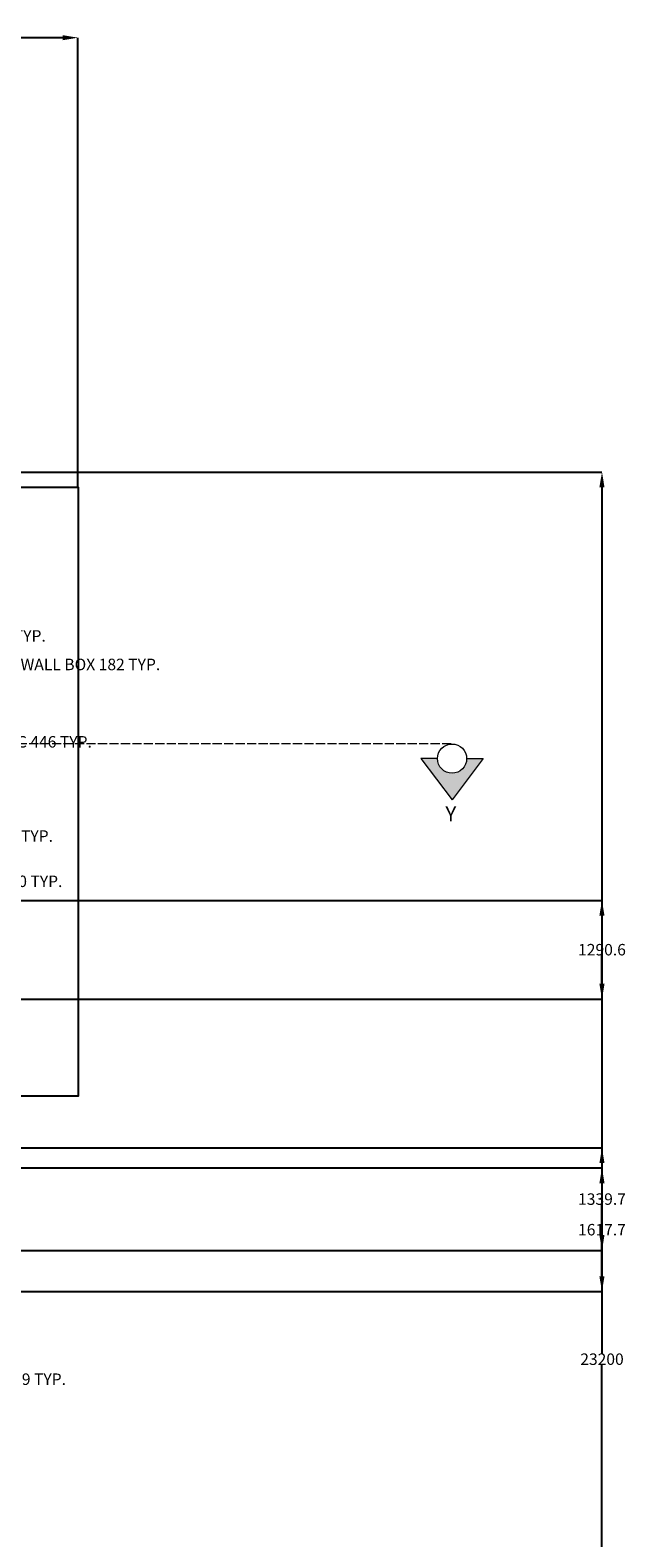
# Model space of a CAD drawing. Units: inches. Extents: x 22626 to 57351, y 2118 to 36234.
# Tile 10 of 10: x 49561 to 57351, y 16521 to 36234. Entities that reach past the tile are written whole.
import ezdxf

# ---------------------------------------------------------------- set-up
doc = ezdxf.new("R2010")
doc.units = ezdxf.units.IN
doc.header["$MEASUREMENT"] = 0
doc.linetypes.add('ACAD_ISO02W100', pattern=[15, 12, -3])
for name, color, linetype, lineweight in [('A-ANNO-DIMS', 130, 'Continuous', 18), ('A-ANNO-SYMB', 130, 'Continuous', 18), ('A-ROOF', 80, 'Continuous', 25)]:
    doc.layers.add(name, color=color, linetype=linetype, lineweight=lineweight)
doc.layers.add('A-SECT', color=2, linetype='ACAD_ISO02W100', lineweight=18, true_color=0xf1eb1f)
doc.styles.get("Standard").update_dxf_attribs({"font": 'arial.ttf'})
doc.dimstyles.get("Standard").update_dxf_attribs({"dimtxt": 150, "dimasz": 200, "dimexe": 0.18, "dimexo": 0.0625, "dimgap": 0.09, "dimtad": 0, "dimtih": 1, "dimtoh": 1, "dimdec": 0, "dimzin": 0, "dimdsep": 46, "dimtxsty": 'Standard', "dimcen": 0.09, "dimadec": 0, "dimazin": 0, "dimtfac": 1, "dimtdec": 0, "dimtofl": 0, "dimtmove": 0, "dimatfit": 3, "dimfxl": 1, "dimtolj": 1, "dimtzin": 0, "dimarcsym": 0})

# ---------------------------------------------------------------- blocks, each defined once
blk = doc.blocks.new('SECTION-HEAD')
h = blk.add_hatch(color=256)
h.dxf.hatch_style = 1
h.paths.add_polyline_path([(815, 541), (599, 541, -1), (216, 541), (0, 541), (407, 0)])
for p, q in [((216, 541), (0, 541)), ((0, 541), (407, 0)), ((815, 541), (407, 0)), ((599, 541), (815, 541))]:
    blk.add_line(p, q)
blk.add_circle((407, 541), 191)
blk = doc.blocks.new('*D62')
at = {"layer": 'A-ANNO-DIMS', "color": 0, "lineweight": -2, "transparency": 16777216}
for p, q in [((48512, 26995), (48512, 26928)), ((48712, 26929), (48757, 26929)), ((48957, 26995), (48957, 26928)), ((48957, 26929), (49157, 26929))]:
    blk.add_line(p, q, dxfattribs=at)
at = {"layer": 'A-ANNO-DIMS', "color": 0, "transparency": 16777216}
for points in [[(48712, 26962), (48712, 26895), (48512, 26929)], [(48757, 26962), (48757, 26895), (48957, 26929)]]:
    blk.add_solid(points, dxfattribs=at)
at = {"layer": 'Defpoints', "color": 0, "transparency": 16777216}
for p in [(48512, 26995), (48957, 26995), (48957, 26929)]:
    blk.add_point(p, dxfattribs=at)
at = {"layer": 'A-ANNO-DIMS', "color": 0, "transparency": 16777216, "insert": (49788, 26929), "char_height": 150, "attachment_point": 5}
blk.add_mtext('\\A1;WC 446 TYP.', dxfattribs=at)
blk = doc.blocks.new('*D64')
at = {"layer": 'A-ANNO-DIMS', "color": 0, "lineweight": -2, "transparency": 16777216}
for p, q in [((48957, 26152), (49094, 26152)), ((49094, 25952), (49094, 25774)), ((49094, 25442), (49094, 25620)), ((48957, 25242), (49094, 25242))]:
    blk.add_line(p, q, dxfattribs=at)
at = {"layer": 'A-ANNO-DIMS', "color": 0, "transparency": 16777216}
for points in [[(49061, 25952), (49127, 25952), (49094, 26152)], [(49061, 25442), (49127, 25442), (49094, 25242)]]:
    blk.add_solid(points, dxfattribs=at)
at = {"layer": 'Defpoints', "color": 0, "transparency": 16777216}
for p in [(48957, 26152), (49094, 26152), (48957, 25242)]:
    blk.add_point(p, dxfattribs=at)
at = {"layer": 'A-ANNO-DIMS', "color": 0, "transparency": 16777216, "insert": (49094, 25697), "char_height": 150, "attachment_point": 5}
blk.add_mtext('\\A1;VANITY 910 TYP.', dxfattribs=at)
blk = doc.blocks.new('*D65')
at = {"layer": 'A-ANNO-DIMS', "color": 0, "lineweight": -2, "transparency": 16777216}
for p, q in [((48348, 25242), (48348, 25105)), ((48957, 25242), (48957, 25105)), ((48548, 25105), (48757, 25105)), ((48957, 25105), (49157, 25105))]:
    blk.add_line(p, q, dxfattribs=at)
at = {"layer": 'A-ANNO-DIMS', "color": 0, "transparency": 16777216}
for points in [[(48548, 25139), (48548, 25072), (48348, 25105)], [(48757, 25139), (48757, 25072), (48957, 25105)]]:
    blk.add_solid(points, dxfattribs=at)
at = {"layer": 'Defpoints', "color": 0, "transparency": 16777216}
for p in [(48348, 25242), (48957, 25242), (48957, 25105)]:
    blk.add_point(p, dxfattribs=at)
at = {"layer": 'A-ANNO-DIMS', "color": 0, "transparency": 16777216, "insert": (49581, 25105), "char_height": 150, "attachment_point": 5}
blk.add_mtext('\\A1;610 TYP.', dxfattribs=at)
blk = doc.blocks.new('*D66')
at = {"layer": 'A-ANNO-DIMS', "color": 0, "lineweight": -2, "transparency": 16777216}
for p, q in [((46732, 18595), (46532, 18595)), ((46932, 18567), (46932, 18595)), ((47122, 18567), (47122, 18595)), ((47322, 18595), (47522, 18595))]:
    blk.add_line(p, q, dxfattribs=at)
at = {"layer": 'A-ANNO-DIMS', "color": 0, "transparency": 16777216}
for points in [[(46732, 18629), (46732, 18562), (46932, 18595)], [(47322, 18629), (47322, 18562), (47122, 18595)]]:
    blk.add_solid(points, dxfattribs=at)
at = {"layer": 'Defpoints', "color": 0, "transparency": 16777216}
for p in [(46932, 18567), (47122, 18595), (47122, 18567)]:
    blk.add_point(p, dxfattribs=at)
at = {"layer": 'A-ANNO-DIMS', "color": 0, "transparency": 16777216, "insert": (48824, 18595), "char_height": 150, "attachment_point": 5}
blk.add_mtext('\\A1;SUPPLY FITTING 189 TYP.', dxfattribs=at)
blk = doc.blocks.new('*D70')
at = {"layer": 'A-ANNO-DIMS', "color": 0, "lineweight": -2, "transparency": 16777216}
for p, q in [((48575, 27941), (48375, 27941)), ((48775, 27914), (48775, 27941)), ((48957, 27914), (48957, 27941)), ((49157, 27941), (49357, 27941))]:
    blk.add_line(p, q, dxfattribs=at)
at = {"layer": 'A-ANNO-DIMS', "color": 0, "transparency": 16777216}
for points in [[(48575, 27974), (48575, 27908), (48775, 27941)], [(49157, 27974), (49157, 27908), (48957, 27941)]]:
    blk.add_solid(points, dxfattribs=at)
at = {"layer": 'Defpoints', "color": 0, "transparency": 16777216}
for p in [(48775, 27914), (48957, 27941), (48957, 27914)]:
    blk.add_point(p, dxfattribs=at)
at = {"layer": 'A-ANNO-DIMS', "color": 0, "transparency": 16777216, "insert": (50349, 27941), "char_height": 150, "attachment_point": 5}
blk.add_mtext('\\A1;WALL BOX 182 TYP.', dxfattribs=at)
blk = doc.blocks.new('*D71')
at = {"layer": 'A-ANNO-DIMS', "color": 0, "lineweight": -2, "transparency": 16777216}
for p, q in [((48748, 28114), (48748, 28314)), ((48748, 28314), (48948, 28314)), ((48775, 27914), (48748, 27914)), ((48775, 27807), (48748, 27807)), ((48748, 27607), (48748, 27407))]:
    blk.add_line(p, q, dxfattribs=at)
at = {"layer": 'A-ANNO-DIMS', "color": 0, "transparency": 16777216}
for points in [[(48715, 28114), (48781, 28114), (48748, 27914)], [(48715, 27607), (48781, 27607), (48748, 27807)]]:
    blk.add_solid(points, dxfattribs=at)
at = {"layer": 'Defpoints', "color": 0, "transparency": 16777216}
for p in [(48748, 27914), (48775, 27914), (48775, 27807)]:
    blk.add_point(p, dxfattribs=at)
at = {"layer": 'A-ANNO-DIMS', "color": 0, "transparency": 16777216, "insert": (49364, 28314), "char_height": 150, "attachment_point": 5}
blk.add_mtext('\\A1;107 TYP.', dxfattribs=at)
blk = doc.blocks.new('*D98')
at = {"layer": 'A-ANNO-DIMS', "color": 0, "lineweight": -2, "transparency": 16777216}
for p, q in [((30057, 30257), (30057, 36136)), ((30257, 36136), (39839, 36136)), ((49987, 36136), (40406, 36136)), ((50187, 30257), (50187, 36136))]:
    blk.add_line(p, q, dxfattribs=at)
at = {"layer": 'A-ANNO-DIMS', "color": 0, "transparency": 16777216}
for points in [[(30257, 36169), (30257, 36103), (30057, 36136)], [(49987, 36169), (49987, 36103), (50187, 36136)]]:
    blk.add_solid(points, dxfattribs=at)
at = {"layer": 'Defpoints', "color": 0, "transparency": 16777216}
for p in [(50187, 36136), (30057, 30257), (50187, 30257)]:
    blk.add_point(p, dxfattribs=at)
at = {"layer": 'A-ANNO-DIMS', "color": 0, "transparency": 16777216, "insert": (40122, 36136), "char_height": 150, "attachment_point": 5}
blk.add_mtext('\\A1;20130', dxfattribs=at)
blk = doc.blocks.new('*D99')
at = {"layer": 'A-ANNO-DIMS', "color": 0, "lineweight": -2, "transparency": 16777216}
for p, q in [((41185, 30457), (57039, 30457)), ((57039, 30257), (57039, 18934)), ((57039, 7457), (57039, 18780)), ((43702, 7257), (57039, 7257))]:
    blk.add_line(p, q, dxfattribs=at)
at = {"layer": 'A-ANNO-DIMS', "color": 0, "transparency": 16777216}
for points in [[(57005, 30257), (57072, 30257), (57039, 30457)], [(57005, 7457), (57072, 7457), (57039, 7257)]]:
    blk.add_solid(points, dxfattribs=at)
at = {"layer": 'Defpoints', "color": 0, "transparency": 16777216}
for p in [(41185, 30457), (57039, 30457), (43702, 7257)]:
    blk.add_point(p, dxfattribs=at)
at = {"layer": 'A-ANNO-DIMS', "color": 0, "transparency": 16777216, "insert": (57039, 18857), "char_height": 150, "attachment_point": 5}
blk.add_mtext('\\A1;23200', dxfattribs=at)
blk = doc.blocks.new('*D103')
at = {"layer": 'A-ANNO-DIMS', "color": 0, "lineweight": -2, "transparency": 16777216}
for p, q in [((42816, 21358), (57039, 21358)), ((57039, 21158), (57039, 20626)), ((57039, 19941), (57039, 20473)), ((42816, 19741), (57039, 19741))]:
    blk.add_line(p, q, dxfattribs=at)
at = {"layer": 'A-ANNO-DIMS', "color": 0, "transparency": 16777216}
for points in [[(57005, 21158), (57072, 21158), (57039, 21358)], [(57005, 19941), (57072, 19941), (57039, 19741)]]:
    blk.add_solid(points, dxfattribs=at)
at = {"layer": 'Defpoints', "color": 0, "transparency": 16777216}
for p in [(42816, 21358), (57039, 21358), (42816, 19741)]:
    blk.add_point(p, dxfattribs=at)
at = {"layer": 'A-ANNO-DIMS', "color": 0, "transparency": 16777216, "insert": (57039, 20550), "char_height": 150, "attachment_point": 5}
blk.add_mtext('\\A1;1617.7', dxfattribs=at)
blk = doc.blocks.new('*D105')
at = {"layer": 'A-ANNO-DIMS', "color": 0, "lineweight": -2, "transparency": 16777216}
for p, q in [((39983, 21620), (57039, 21620)), ((57039, 21420), (57039, 21027)), ((57039, 20480), (57039, 20874)), ((39983, 20280), (57039, 20280))]:
    blk.add_line(p, q, dxfattribs=at)
at = {"layer": 'A-ANNO-DIMS', "color": 0, "transparency": 16777216}
for points in [[(57005, 21420), (57072, 21420), (57039, 21620)], [(57005, 20480), (57072, 20480), (57039, 20280)]]:
    blk.add_solid(points, dxfattribs=at)
at = {"layer": 'Defpoints', "color": 0, "transparency": 16777216}
for p in [(39983, 21620), (57039, 21620), (39983, 20280)]:
    blk.add_point(p, dxfattribs=at)
at = {"layer": 'A-ANNO-DIMS', "color": 0, "transparency": 16777216, "insert": (57039, 20950), "char_height": 150, "attachment_point": 5}
blk.add_mtext('\\A1;1339.7', dxfattribs=at)
blk = doc.blocks.new('*D109')
at = {"layer": 'A-ANNO-DIMS', "color": 0, "lineweight": -2, "transparency": 16777216}
for p, q in [((38641, 24856), (57039, 24856)), ((57039, 24656), (57039, 24287)), ((57039, 23765), (57039, 24134)), ((38641, 23565), (57039, 23565))]:
    blk.add_line(p, q, dxfattribs=at)
at = {"layer": 'A-ANNO-DIMS', "color": 0, "transparency": 16777216}
for points in [[(57005, 24656), (57072, 24656), (57039, 24856)], [(57005, 23765), (57072, 23765), (57039, 23565)]]:
    blk.add_solid(points, dxfattribs=at)
at = {"layer": 'Defpoints', "color": 0, "transparency": 16777216}
for p in [(38641, 24856), (57039, 24856), (38641, 23565)]:
    blk.add_point(p, dxfattribs=at)
at = {"layer": 'A-ANNO-DIMS', "color": 0, "transparency": 16777216, "insert": (57039, 24211), "char_height": 150, "attachment_point": 5}
blk.add_mtext('\\A1;1290.6', dxfattribs=at)
blk = doc.blocks.new('*D115')
at = {"layer": 'A-ANNO-DIMS', "color": 0, "lineweight": -2, "transparency": 16777216}
for p, q in [((47973, 25697), (48173, 25697)), ((49783, 25697), (49783, 25697)), ((49783, 25697), (49783, 25697))]:
    blk.add_line(p, q, dxfattribs=at)
at = {"layer": 'A-ANNO-DIMS', "color": 0, "transparency": 16777216}
blk.add_solid([(48173, 25730), (48173, 25664), (48373, 25697)], dxfattribs=at)
at = {"layer": 'Defpoints', "color": 0, "transparency": 16777216}
for p in [(48373, 25697), (49783, 25697)]:
    blk.add_point(p, dxfattribs=at)
at = {"layer": 'A-ANNO-DIMS', "color": 0, "transparency": 16777216, "insert": (47515, 25697), "char_height": 150, "attachment_point": 5}
blk.add_mtext('\\A1;2X R1410', dxfattribs=at)

msp = doc.modelspace()

# ---------------------------------------------------------------- linework, layer by layer
at = {"layer": 'A-ROOF'}
msp.add_lwpolyline([(41184.53, 30256.86), (50187.43, 30256.86), (50187.43, 25126.86), (50187.43, 22296.86), (48682.43, 22296.86), (48682.43, 11956.86), (43702.43, 11956.86)], dxfattribs=at)
at = {"layer": 'A-SECT', "ltscale": 10}
msp.add_line((55067.61, 26900.74), (24870.06, 26900.74), dxfattribs=at)

# ---------------------------------------------------------------- block references
at = {"layer": 'A-ANNO-SYMB'}
msp.add_blockref('SECTION-HEAD', (54671.15, 26168.47), dxfattribs=at)

# ---------------------------------------------------------------- texts
msp.add_text('Y', height=200, dxfattribs=at).set_placement((54989.81, 25887.63))

# ---------------------------------------------------------------- dimensions: what is measured, and where the dimension line sits
at = {"layer": 'A-ANNO-DIMS'}
dim = msp.add_linear_dim(base=(50187.43, 36136.06), p1=(30057.43, 30256.86), p2=(50187.43, 30256.86), dimstyle='Standard', override={"dimdec": 0, "dimlfac": 1, "dimrnd": 0, "dimzin": 0, "dimdsep": 46, "dimlunit": 2}, dxfattribs=at)
dim.commit()
dim.dimension.update_dxf_attribs({"geometry": '*D98', "text_midpoint": (40122.43, 36136.06)})
for base, p1, p2, override, picture, middle in [((57038.61, 30456.86), (43702.43, 7256.86), (41184.53, 30456.86), {"dimdec": 0, "dimlfac": 1, "dimrnd": 0, "dimzin": 0, "dimdsep": 46, "dimlunit": 2}, '*D99', (57038.61, 18856.86)), ((57038.61, 24856.11), (38641.03, 23565.5), (38641.03, 24856.11), {"dimdec": 1, "dimlfac": 1, "dimrnd": 0, "dimzin": 0, "dimdsep": 46, "dimlunit": 2}, '*D109', (57038.61, 24210.8)), ((57038.61, 21620.09), (39982.98, 20280.39), (39982.98, 21620.09), {"dimdec": 1, "dimlfac": 1, "dimrnd": 0, "dimzin": 0, "dimdsep": 46, "dimlunit": 2}, '*D105', (57038.61, 20950.24)), ((57038.6134, 21358.3711), (42815.7406, 19740.7168), (42815.7406, 21358.3711), {"dimdec": 1, "dimlfac": 1, "dimrnd": 0, "dimzin": 0, "dimdsep": 46, "dimlunit": 2}, '*D103', (57038.6134, 20549.5439))]:
    dim = msp.add_linear_dim(base=base, p1=p1, p2=p2, angle=90, dimstyle='Standard', override=override, dxfattribs=at)
    dim.commit()
    dim.dimension.update_dxf_attribs({"geometry": picture, "text_midpoint": middle})
for base, p1, p2, text, picture, middle in [((48957.43, 27941), (48775.41, 27913.69), (48957.43, 27913.69), 'WALL BOX <> TYP.', '*D70', (50348.74, 27941)), ((48957.43, 26928.62), (48511.9, 26995.45), (48957.43, 26995.45), 'WC <> TYP.', '*D62', (49787.6, 26928.62)), ((48957.43, 25105.35), (48347.56, 25241.86), (48957.43, 25241.86), '<> TYP.', '*D65', (49581.27, 25105.35)), ((47121.6, 18595.27), (46932.22, 18566.86), (47121.6, 18566.86), 'SUPPLY FITTING <> TYP.', '*D66', (48823.75, 18595.27))]:
    dim = msp.add_linear_dim(base=base, p1=p1, p2=p2, text=text, dimstyle='Standard', override={"dimdec": 0, "dimlfac": 1, "dimrnd": 0, "dimzin": 0, "dimdsep": 46, "dimlunit": 2}, dxfattribs=at)
    dim.commit()
    dim.dimension.update_dxf_attribs({"geometry": picture, "text_midpoint": middle})
for base, p1, p2, text, picture, middle in [((48748.11, 27913.69), (48775.41, 27806.86), (48775.41, 27913.69), '<> TYP.', '*D71', (49364.48, 28313.69)), ((49093.94, 26151.9), (48957.43, 25241.86), (48957.43, 26151.9), 'VANITY <> TYP.', '*D64', (49093.94, 25696.88))]:
    dim = msp.add_linear_dim(base=base, p1=p1, p2=p2, angle=90, text=text, dimstyle='Standard', override={"dimdec": 0, "dimlfac": 1, "dimrnd": 0, "dimzin": 0, "dimdsep": 46, "dimlunit": 2}, dxfattribs=at)
    dim.commit()
    dim.dimension.update_dxf_attribs({"geometry": picture, "text_midpoint": middle})
dim = msp.add_radius_dim(center=(49782.7, 25696.88), mpoint=(48372.71, 25696.88), text='2X <>', dimstyle='Standard', override={"dimdec": 0, "dimlfac": 1, "dimrnd": 0, "dimzin": 0, "dimdsep": 46, "dimlunit": 2}, dxfattribs=at)
dim.commit()
dim.dimension.update_dxf_attribs({"geometry": '*D115', "text_midpoint": (47514.69, 25696.88)})

doc.saveas('drawing.dxf')
